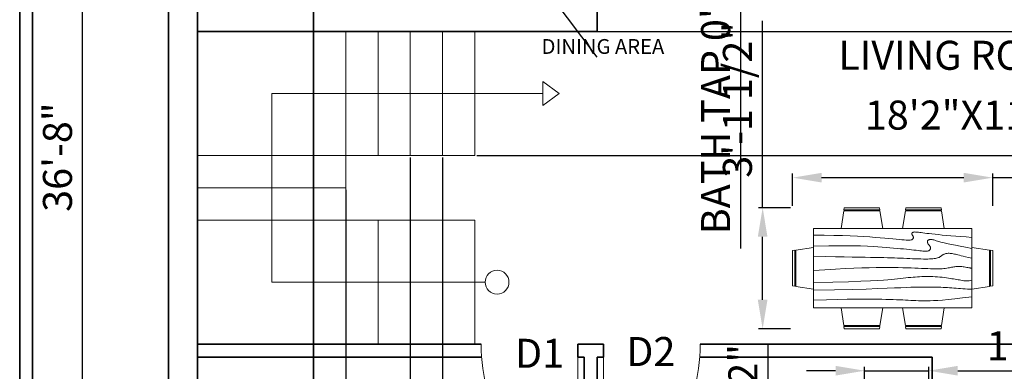
# Model space of a CAD drawing. Units: inches. Extents: x 2436 to 3928, y 1526 to 2149.
# Tile 2 of 6: x 2436 to 2742, y 1731 to 1840. Entities that reach past the tile are written whole.
import ezdxf

# ---------------------------------------------------------------- set-up
doc = ezdxf.new("R2010")
doc.units = ezdxf.units.IN
for name, color, linetype, lineweight in [('A-ANNO-SYMB', 7, 'Continuous', 13), ('A-AREA-IDEN', 152, 'Continuous', 18), ('A-DOOR', 4, 'Continuous', 18), ('A-DOOR-TEXT', 30, 'Continuous', 18), ('A-FLOR-STRS', 7, 'Continuous', 18), ('A-FURN', 8, 'Continuous', 18), ('A-WALL', 7, 'Continuous', 35), ('G-ANNO-TTLB', 7, 'Continuous', 35), ('S-ANNO-DIMS', 2, 'Continuous', 18)]:
    doc.layers.add(name, color=color, linetype=linetype, lineweight=lineweight)
doc.styles.get("Standard").update_dxf_attribs({"font": 'arial.ttf'})
doc.dimstyles.new('ISO-25', dxfattribs={"dimtxt": 9, "dimasz": 9, "dimexe": 1.25, "dimexo": 0.625, "dimgap": 2, "dimtad": 1, "dimdec": 1, "dimlunit": 4, "dimtxsty": 'Standard', "dimcen": 2.5, "dimadec": 0, "dimazin": 0, "dimtfac": 1, "dimtdec": 1, "dimtmove": 0, "dimatfit": 3, "dimfxl": 1, "dimarcsym": 0})

# ---------------------------------------------------------------- blocks, each defined once
blk = doc.blocks.new('Dining Set - 36 x 72 in.')
for p, q in [((-22, 27.5), (-22.1562, 26.50042)), ((-22, 27.5), (-6, 27.5)), ((-5.8437, 26.49966), (-6, 27.5)), ((6, 27.5), (5.8438, 26.50042)), ((6, 27.5), (22, 27.5)), ((22.1563, 26.49966), (22, 27.5)), ((-22.2343, 26.00059), (-23.4847, 17.99762)), ((-22.2304, 26), (-5.7608, 26)), ((-5.8416, 26.5), (-22.1534, 26.5)), ((-4.5152, 17.99762), (-5.7655, 25.99926)), ((5.7657, 26.00059), (4.5153, 17.99762)), ((5.7696, 26), (22.2392, 26)), ((22.1584, 26.5), (5.8466, 26.5)), ((23.4848, 17.99762), (22.2345, 25.99926)), ((36, 18), (-36, 18)), ((-36, 18), (-36, -18)), ((36, -18), (36, 18)), ((-44.0006, 8.23428), (-35.9976, 9.48474)), ((44.0006, 8.23428), (35.9976, 9.48474)), ((-45.5, 8), (-44.5004, 8.15617)), ((-45.5, 8), (-45.5, -8)), ((-44.5, -8.15843), (-44.5, 8.15338)), ((-44, 8.23041), (-44, -8.23915)), ((44, 8.23041), (44, -8.23915)), ((44.5, -8.15843), (44.5, 8.15338)), ((45.5, 8), (44.5005, 8.15617)), ((45.5, 8), (45.5, -8)), ((-44.4997, -8.15631), (-45.5, -8)), ((-35.9976, -9.48476), (-43.9993, -8.2345)), ((35.9976, -9.48476), (43.9993, -8.2345)), ((44.4997, -8.15631), (45.5, -8)), ((-36, -18), (36, -18)), ((-22.2343, -26.0006), (-23.4847, -17.99762)), ((-4.5152, -17.99762), (-5.7655, -25.99928)), ((5.7657, -26.0006), (4.5153, -17.99762)), ((23.4848, -17.99762), (22.2345, -25.99928)), ((-22.2304, -26), (-5.7608, -26)), ((-22, -27.5), (-22.1562, -26.50044)), ((-5.8416, -26.5), (-22.1534, -26.5)), ((-5.8437, -26.49967), (-6, -27.5)), ((5.7696, -26), (22.2392, -26)), ((6, -27.5), (5.8438, -26.50044)), ((22.1584, -26.5), (5.8466, -26.5)), ((22.1563, -26.49967), (22, -27.5)), ((-22, -27.5), (-6, -27.5)), ((6, -27.5), (22, -27.5))]:
    blk.add_line(p, q)
for points in [[(-36, 15), (-31.1772, 14.97754), (-26.8079, 14.91406), (-22.8538, 14.81543), (-19.276, 14.6875), (-16.0362, 14.53613), (-13.0957, 14.36718), (-10.4159, 14.18652), (-7.9583, 14), (-5.6904, 13.81315), (-3.6035, 13.63021), (-1.6954, 13.45508), (0.0365, 13.29166), (1.5945, 13.14388), (2.9811, 13.01562), (4.1988, 12.9108), (5.25, 12.83333), (6.1393, 12.78613), (6.8802, 12.76823), (7.4883, 12.77767), (7.9792, 12.8125), (8.3685, 12.87077), (8.6719, 12.95052), (8.9049, 13.0498), (9.0833, 13.16666), (9.2205, 13.29899), (9.3216, 13.44401), (9.3895, 13.59879), (9.4271, 13.76041), (9.4373, 13.92594), (9.4232, 14.09245), (9.3875, 14.257), (9.3333, 14.41666), (9.2638, 14.56917), (9.1836, 14.71484), (9.0975, 14.85465), (9.0104, 14.98958), (8.9272, 15.1206), (8.8529, 15.2487), (8.7922, 15.37483), (8.75, 15.5), (8.7305, 15.62467), (8.7344, 15.74739), (8.7617, 15.86621), (8.8125, 15.97916), (8.8867, 16.08431), (8.9844, 16.17968), (9.1055, 16.26334), (9.25, 16.33333), (9.4189, 16.38802), (9.6172, 16.42708), (9.8506, 16.45052), (10.125, 16.45833), (10.4463, 16.45052), (10.8203, 16.42708), (11.2529, 16.38802), (11.75, 16.33333), (12.3184, 16.26318), (12.9694, 16.17838), (13.7151, 16.07991), (14.5677, 15.96875), (15.5395, 15.84586), (16.6426, 15.71224), (17.8893, 15.56884), (19.2917, 15.41666), (20.859, 15.25667), (22.5879, 15.08984), (24.4721, 14.91715), (26.5052, 14.73958), (28.6809, 14.5581), (30.9929, 14.3737), (33.4347, 14.18733), (36, 14)], [(-36, 10), (-28.9766, 10.14274), (-23.1725, 10.20442), (-18.4241, 10.19775), (-14.5677, 10.13541), (-11.4399, 10.03011), (-8.877, 9.89453), (-6.7154, 9.74137), (-4.7917, 9.58333), (-2.9698, 9.43082), (-1.2246, 9.28515), (0.4415, 9.14534), (2.026, 9.01041), (3.5266, 8.87939), (4.9408, 8.7513), (6.266, 8.62516), (7.5, 8.5), (8.6411, 8.37549), (9.6914, 8.2539), (10.6538, 8.13818), (11.5312, 8.03125), (12.3267, 7.93603), (13.043, 7.85547), (13.6831, 7.79248), (14.25, 7.75), (14.7471, 7.7303), (15.1797, 7.73307), (15.5537, 7.75732), (15.875, 7.80208), (16.1494, 7.86637), (16.3828, 7.94922), (16.5811, 8.04964), (16.75, 8.16666), (16.8944, 8.29915), (17.0143, 8.44531), (17.1089, 8.60319), (17.1771, 8.77083), (17.218, 8.94629), (17.2305, 9.1276), (17.2137, 9.31282), (17.1667, 9.5), (17.0895, 9.6875), (16.987, 9.875), (16.8649, 10.0625), (16.7292, 10.25), (16.5856, 10.4375), (16.4401, 10.625), (16.2985, 10.8125), (16.1667, 11), (16.05, 11.18733), (15.9518, 11.3737), (15.8752, 11.5581), (15.8229, 11.73958), (15.798, 11.91715), (15.8034, 12.08984), (15.842, 12.25667), (15.9167, 12.41666), (16.0295, 12.56836), (16.1784, 12.70833), (16.3605, 12.83268), (16.5729, 12.9375), (16.8127, 13.01888), (17.0768, 13.07291), (17.3625, 13.0957), (17.6667, 13.08333), (17.9894, 13.03312), (18.3418, 12.94726), (18.7382, 12.82918), (19.1927, 12.68229), (19.7195, 12.51001), (20.3327, 12.31575), (21.0465, 12.10294), (21.875, 11.875), (22.8357, 11.63354), (23.959, 11.37304), (25.2786, 11.08618), (26.8282, 10.76562), (28.6414, 10.40405), (30.752, 9.99414), (33.1936, 9.52856), (36, 9)], [(-36, 5.5), (-30.7157, 5.3348), (-26.069, 5.20963), (-21.9946, 5.11767), (-18.4271, 5.05208), (-15.3009, 5.00602), (-12.5508, 4.97265), (-10.1112, 4.94515), (-7.9167, 4.91666), (-5.909, 4.88167), (-4.0586, 4.83984), (-2.3429, 4.79215), (-0.7396, 4.73958), (0.7739, 4.6831), (2.22, 4.6237), (3.6213, 4.56233), (5, 4.5), (6.373, 4.43782), (7.7344, 4.3776), (9.0723, 4.32129), (10.375, 4.27083), (11.6309, 4.22819), (12.8281, 4.19531), (13.9551, 4.17415), (15, 4.16666), (15.954, 4.17448), (16.819, 4.19791), (17.6001, 4.23698), (18.3021, 4.29166), (18.9299, 4.36198), (19.4883, 4.44791), (19.9823, 4.54948), (20.4167, 4.66666), (20.7969, 4.79899), (21.1302, 4.94401), (21.4245, 5.09879), (21.6875, 5.26041), (21.9271, 5.42594), (22.1511, 5.59245), (22.3672, 5.757), (22.5834, 5.91666), (22.8065, 6.06868), (23.0404, 6.21093), (23.2879, 6.34147), (23.5521, 6.45833), (23.8358, 6.55957), (24.142, 6.64323), (24.4735, 6.70735), (24.8334, 6.75), (25.2235, 6.76969), (25.642, 6.76692), (26.0858, 6.74267), (26.5521, 6.69791), (27.0379, 6.63362), (27.5404, 6.55078), (28.0565, 6.45036), (28.5834, 6.33333), (29.1242, 6.19987), (29.7071, 6.04687), (30.3661, 5.87044), (31.1354, 5.66666), (32.0493, 5.43164), (33.142, 5.16146), (34.4475, 4.85221), (36, 4.5)], [(-36, -1), (-30.7915, -0.6591), (-26.0195, -0.38216), (-21.6519, -0.16284), (-17.6563, 0.00521), (-14.0005, 0.12833), (-10.6523, 0.21289), (-7.5796, 0.26522), (-4.75, 0.29166), (-2.134, 0.29793), (0.2878, 0.28711), (2.5317, 0.26163), (4.6146, 0.22396), (6.5529, 0.17651), (8.3633, 0.12174), (10.0623, 0.06209), (11.6667, 0), (13.1899, -0.06201), (14.6341, -0.1211), (15.9982, -0.17432), (17.2813, -0.21875), (18.4823, -0.25147), (19.6003, -0.26953), (20.6343, -0.27002), (21.5834, -0.25), (22.4481, -0.20768), (23.2357, -0.14584), (23.9549, -0.06836), (24.6146, 0.02083), (25.2235, 0.11784), (25.7904, 0.21875), (26.3241, 0.31966), (26.8334, 0.41666), (27.3265, 0.50618), (27.8099, 0.58593), (28.2894, 0.65397), (28.7709, 0.70833), (29.2601, 0.74707), (29.763, 0.76823), (30.2855, 0.76985), (30.8334, 0.75), (31.4088, 0.70784), (31.9994, 0.64713), (32.589, 0.57275), (33.1615, 0.48958), (33.7008, 0.4025), (34.1908, 0.3164), (34.6153, 0.23616), (34.9584, 0.16666), (35.2099, 0.11165), (35.3848, 0.07031), (35.504, 0.04069), (35.5886, 0.02083), (35.6594, 0.00879), (35.7377, 0.0026), (35.8442, 0.00032), (36, 0)], [(-36, -6.5), (-27.1843, -6.31267), (-20.084, -6.1263), (-14.469, -5.9419), (-10.1094, -5.76042), (-6.7752, -5.58285), (-4.2363, -5.41016), (-2.2629, -5.24333), (-0.625, -5.08334), (0.8708, -4.93099), (2.2715, -4.78646), (3.5872, -4.64974), (4.8281, -4.52084), (6.0046, -4.39974), (7.127, -4.28646), (8.2053, -4.18099), (9.25, -4.08334), (10.2705, -3.99382), (11.2734, -3.91407), (12.2647, -3.84603), (13.25, -3.79167), (14.2354, -3.75293), (15.2266, -3.73177), (16.2295, -3.73015), (17.25, -3.75), (18.2912, -3.79248), (19.3451, -3.85547), (20.4009, -3.93604), (21.4479, -4.03125), (22.4754, -4.13819), (23.4727, -4.25391), (24.4289, -4.37549), (25.3334, -4.5), (26.1785, -4.62492), (26.9694, -4.74935), (27.7145, -4.87281), (28.4219, -4.99479), (29.1, -5.11483), (29.7572, -5.23242), (30.4016, -5.34709), (31.0417, -5.45834), (31.6837, -5.56437), (32.3262, -5.65821), (32.9658, -5.73153), (33.599, -5.77604), (34.2224, -5.78345), (34.8327, -5.74545), (35.4264, -5.65373), (36, -5.5)], [(-36, -10), (-26.4022, -9.81299), (-18.4675, -9.62891), (-11.9839, -9.45069), (-6.7396, -9.28125), (-2.5226, -9.12354), (0.8789, -8.98047), (3.6769, -8.85498), (6.0833, -8.75), (8.2767, -8.66765), (10.3021, -8.60677), (12.1712, -8.56543), (13.8958, -8.54167), (15.4876, -8.53353), (16.9583, -8.53907), (18.3197, -8.55632), (19.5834, -8.58334), (20.7616, -8.61841), (21.8685, -8.66081), (22.9188, -8.71004), (23.9271, -8.76563), (24.9081, -8.82707), (25.8763, -8.89388), (26.8465, -8.96558), (27.8334, -9.04167), (28.8474, -9.12118), (29.8828, -9.20117), (30.93, -9.27824), (31.9792, -9.34896), (33.0205, -9.40991), (34.0443, -9.45768), (35.0407, -9.48885), (36, -9.5)], [(-36, -14.5), (-30.0881, -14.33513), (-25.0332, -14.21224), (-20.7312, -14.12647), (-17.0781, -14.07292), (-13.97, -14.04671), (-11.3027, -14.04297), (-8.9724, -14.05681), (-6.875, -14.08334), (-4.9224, -14.11833), (-3.0905, -14.16016), (-1.3709, -14.20785), (0.2448, -14.26042), (1.7647, -14.3169), (3.1973, -14.3763), (4.5507, -14.43767), (5.8333, -14.5), (7.0554, -14.5621), (8.235, -14.62175), (9.3922, -14.67652), (10.5469, -14.72396), (11.7192, -14.76164), (12.929, -14.78711), (14.1965, -14.79794), (15.5417, -14.79167), (16.9933, -14.76424), (18.6152, -14.70508), (20.4804, -14.60197), (22.6615, -14.44271), (25.2312, -14.21509), (28.2624, -13.9069), (31.8277, -13.50594), (36, -13)]]:
    blk.add_lwpolyline(points)
blk = doc.blocks.new('DOOR-SINGLE-30-PLAN')
blk.add_line((0, 0), (0, 48))
blk.add_arc((-23.4, 0), 53.4, 0, 64.0108)
blk = doc.blocks.new('*D42')
at = {"layer": 'Defpoints', "color": 0, "transparency": 16777216}
for p in [(2658.27, 1927.9), (2658.27, 1917.9), (2659.77, 1917.9)]:
    blk.add_point(p, dxfattribs=at)
at = {"layer": 'S-ANNO-DIMS', "color": 0, "lineweight": -2, "transparency": 16777216}
for p, q in [((2659.77, 1936.9), (2659.77, 1945.9)), ((2658.9, 1927.9), (2661.02, 1927.9)), ((2659.77, 1927.9), (2659.77, 1917.9)), ((2658.9, 1917.9), (2661.02, 1917.9)), ((2659.77, 1908.9), (2659.77, 1769.48))]:
    blk.add_line(p, q, dxfattribs=at)
at = {"layer": 'S-ANNO-DIMS', "color": 0, "transparency": 16777216}
for points in [[(2658.27, 1936.9), (2661.27, 1936.9), (2659.77, 1927.9)], [(2658.27, 1908.9), (2661.27, 1908.9), (2659.77, 1917.9)]]:
    blk.add_solid(points, dxfattribs=at)
at = {"layer": 'S-ANNO-DIMS', "color": 0, "transparency": 16777216, "insert": (2653.18, 1834.69), "char_height": 9, "attachment_point": 5, "rotation": 90}
blk.add_mtext('BATH TAP 0\'-10" TYP.', dxfattribs=at)
blk = doc.blocks.new('*D48')
at = {"layer": 'Defpoints', "color": 0, "transparency": 16777216}
for p in [(2738.03, 1791.43), (2675.93, 1782.12), (2738.03, 1782.12)]:
    blk.add_point(p, dxfattribs=at)
at = {"layer": 'S-ANNO-DIMS', "color": 0, "lineweight": -2, "transparency": 16777216}
for p, q in [((2675.93, 1782.74), (2675.93, 1792.68)), ((2684.93, 1791.43), (2729.03, 1791.43)), ((2738.03, 1782.74), (2738.03, 1792.68)), ((2738.03, 1791.43), (2849.95, 1791.43))]:
    blk.add_line(p, q, dxfattribs=at)
at = {"layer": 'S-ANNO-DIMS', "color": 0, "transparency": 16777216}
for points in [[(2684.93, 1792.93), (2684.93, 1789.93), (2675.93, 1791.43)], [(2729.03, 1792.93), (2729.03, 1789.93), (2738.03, 1791.43)]]:
    blk.add_solid(points, dxfattribs=at)
at = {"layer": 'S-ANNO-DIMS', "color": 0, "transparency": 16777216, "insert": (2798.49, 1798.08), "char_height": 9, "attachment_point": 5}
blk.add_mtext('DINING SET 5\'-2"', dxfattribs=at)
blk = doc.blocks.new('*D49')
at = {"layer": 'Defpoints', "color": 0, "transparency": 16777216}
for p in [(2666.62, 1782.12), (2675.93, 1782.12), (2675.93, 1744.58)]:
    blk.add_point(p, dxfattribs=at)
at = {"layer": 'S-ANNO-DIMS', "color": 0, "lineweight": -2, "transparency": 16777216}
for p, q in [((2666.62, 1782.12), (2666.62, 1840.01)), ((2675.31, 1782.12), (2665.37, 1782.12)), ((2666.62, 1753.58), (2666.62, 1773.12)), ((2675.31, 1744.58), (2665.37, 1744.58))]:
    blk.add_line(p, q, dxfattribs=at)
at = {"layer": 'S-ANNO-DIMS', "color": 0, "transparency": 16777216}
for points in [[(2665.12, 1773.12), (2668.12, 1773.12), (2666.62, 1782.12)], [(2665.12, 1753.58), (2668.12, 1753.58), (2666.62, 1744.58)]]:
    blk.add_solid(points, dxfattribs=at)
at = {"layer": 'S-ANNO-DIMS', "color": 0, "transparency": 16777216, "insert": (2659.96, 1815.56), "char_height": 9, "attachment_point": 5, "rotation": 90}
blk.add_mtext('3\'-1 1/2"', dxfattribs=at)
blk = doc.blocks.new('*D51')
at = {"layer": 'Defpoints', "color": 0, "transparency": 16777216}
for p in [(2664.4, 1675.79), (2668.31, 1675.79), (2664.4, 1653.19)]:
    blk.add_point(p, dxfattribs=at)
at = {"layer": 'S-ANNO-DIMS', "color": 0, "lineweight": -2, "transparency": 16777216}
for p, q in [((2668.31, 1675.79), (2668.31, 1739.83)), ((2665.03, 1675.79), (2669.56, 1675.79)), ((2668.31, 1662.19), (2668.31, 1666.79)), ((2665.03, 1653.19), (2669.56, 1653.19))]:
    blk.add_line(p, q, dxfattribs=at)
at = {"layer": 'S-ANNO-DIMS', "color": 0, "transparency": 16777216}
for points in [[(2666.81, 1666.79), (2669.81, 1666.79), (2668.31, 1675.79)], [(2666.81, 1662.19), (2669.81, 1662.19), (2668.31, 1653.19)]]:
    blk.add_solid(points, dxfattribs=at)
at = {"layer": 'S-ANNO-DIMS', "color": 0, "transparency": 16777216, "insert": (2661.66, 1712.31), "char_height": 9, "attachment_point": 5, "rotation": 90}
blk.add_mtext('1\'-10 1/2"', dxfattribs=at)
blk = doc.blocks.new('*D55')
at = {"layer": 'Defpoints', "color": 0, "transparency": 16777216}
for p in [(2718.2, 1731.57), (2698.27, 1727.86), (2718.2, 1727.86)]:
    blk.add_point(p, dxfattribs=at)
at = {"layer": 'S-ANNO-DIMS', "color": 0, "lineweight": -2, "transparency": 16777216}
for p, q in [((2689.27, 1731.57), (2680.27, 1731.57)), ((2698.27, 1728.48), (2698.27, 1732.82)), ((2698.27, 1731.57), (2718.2, 1731.57)), ((2718.2, 1728.48), (2718.2, 1732.82)), ((2727.2, 1731.57), (2763.27, 1731.57))]:
    blk.add_line(p, q, dxfattribs=at)
at = {"layer": 'S-ANNO-DIMS', "color": 0, "transparency": 16777216}
for points in [[(2689.27, 1733.07), (2689.27, 1730.07), (2698.27, 1731.57)], [(2727.2, 1733.07), (2727.2, 1730.07), (2718.2, 1731.57)]]:
    blk.add_solid(points, dxfattribs=at)
at = {"layer": 'S-ANNO-DIMS', "color": 0, "transparency": 16777216, "insert": (2749.73, 1738.16), "char_height": 9, "attachment_point": 5}
blk.add_mtext('1\'-8"', dxfattribs=at)
blk = doc.blocks.new('*D57')
at = {"layer": 'Defpoints', "color": 0, "transparency": 16777216}
for p in [(2455.49, 2017.79), (2482.24, 2017.79), (2482.24, 1577.79)]:
    blk.add_point(p, dxfattribs=at)
at = {"layer": 'S-ANNO-DIMS', "color": 0, "lineweight": -2, "transparency": 16777216}
for p, q in [((2481.61, 2017.79), (2454.24, 2017.79)), ((2455.49, 1586.79), (2455.49, 2008.79)), ((2481.61, 1577.79), (2454.24, 1577.79))]:
    blk.add_line(p, q, dxfattribs=at)
at = {"layer": 'S-ANNO-DIMS', "color": 0, "transparency": 16777216}
for points in [[(2453.99, 2008.79), (2456.99, 2008.79), (2455.49, 2017.79)], [(2453.99, 1586.79), (2456.99, 1586.79), (2455.49, 1577.79)]]:
    blk.add_solid(points, dxfattribs=at)
at = {"layer": 'S-ANNO-DIMS', "color": 0, "transparency": 16777216, "insert": (2448.89, 1797.79), "char_height": 9, "attachment_point": 5, "rotation": 90}
blk.add_mtext('36\'-8"', dxfattribs=at)
blk = doc.blocks.new('*D58')
at = {"layer": 'Defpoints', "color": 0, "transparency": 16777216}
for p in [(2491.24, 2008.79), (2527.24, 2008.79), (2527.24, 1551.04)]:
    blk.add_point(p, dxfattribs=at)
at = {"layer": 'S-ANNO-DIMS', "color": 0, "lineweight": -2, "transparency": 16777216}
for p, q in [((2491.24, 2008.16), (2491.24, 1549.79)), ((2527.24, 2008.16), (2527.24, 1549.79)), ((2500.24, 1551.04), (2518.24, 1551.04))]:
    blk.add_line(p, q, dxfattribs=at)
at = {"layer": 'S-ANNO-DIMS', "color": 0, "transparency": 16777216}
for points in [[(2500.24, 1552.54), (2500.24, 1549.54), (2491.24, 1551.04)], [(2518.24, 1552.54), (2518.24, 1549.54), (2527.24, 1551.04)]]:
    blk.add_solid(points, dxfattribs=at)
at = {"layer": 'S-ANNO-DIMS', "color": 0, "transparency": 16777216, "insert": (2509.24, 1557.64), "char_height": 9, "attachment_point": 5}
blk.add_mtext('3\'-0"', dxfattribs=at)
blk = doc.blocks.new('*D64')
at = {"layer": 'Defpoints', "color": 0, "transparency": 16777216}
for p in [(2527.24, 2114.67), (2491.24, 1603.79), (2527.24, 1603.79)]:
    blk.add_point(p, dxfattribs=at)
at = {"layer": 'S-ANNO-DIMS', "color": 0, "lineweight": -2, "transparency": 16777216}
for p, q in [((2491.24, 1604.41), (2491.24, 2115.92)), ((2527.24, 1604.41), (2527.24, 2115.92)), ((2500.24, 2114.67), (2518.24, 2114.67))]:
    blk.add_line(p, q, dxfattribs=at)
at = {"layer": 'S-ANNO-DIMS', "color": 0, "transparency": 16777216}
for points in [[(2500.24, 2116.17), (2500.24, 2113.17), (2491.24, 2114.67)], [(2518.24, 2116.17), (2518.24, 2113.17), (2527.24, 2114.67)]]:
    blk.add_solid(points, dxfattribs=at)
at = {"layer": 'S-ANNO-DIMS', "color": 0, "transparency": 16777216, "insert": (2509.24, 2121.27), "char_height": 9, "attachment_point": 5}
blk.add_mtext('3\'-0"', dxfattribs=at)
blk = doc.blocks.new('*D71')
at = {"layer": 'Defpoints', "color": 0, "transparency": 16777216}
for p in [(2577.24, 1836.79), (2868.99, 1836.79), (2577.24, 1798.29)]:
    blk.add_point(p, dxfattribs=at)
at = {"layer": 'S-ANNO-DIMS', "color": 0, "lineweight": -2, "transparency": 16777216}
for p, q in [((2868.99, 1836.79), (2868.99, 1894.68)), ((2577.86, 1836.79), (2870.24, 1836.79)), ((2868.99, 1807.29), (2868.99, 1827.79)), ((2577.86, 1798.29), (2870.24, 1798.29))]:
    blk.add_line(p, q, dxfattribs=at)
at = {"layer": 'S-ANNO-DIMS', "color": 0, "transparency": 16777216}
for points in [[(2867.49, 1827.79), (2870.49, 1827.79), (2868.99, 1836.79)], [(2867.49, 1807.29), (2870.49, 1807.29), (2868.99, 1798.29)]]:
    blk.add_solid(points, dxfattribs=at)
at = {"layer": 'S-ANNO-DIMS', "color": 0, "transparency": 16777216, "insert": (2862.33, 1870.23), "char_height": 9, "attachment_point": 5, "rotation": 90}
blk.add_mtext('3\'-2 1/2"', dxfattribs=at)
blk = doc.blocks.new('*D72')
at = {"layer": 'Defpoints', "color": 0, "transparency": 16777216}
for p in [(2491.24, 1798.29), (2537.24, 1788.29), (2537.24, 1551.04)]:
    blk.add_point(p, dxfattribs=at)
at = {"layer": 'S-ANNO-DIMS', "color": 0, "lineweight": -2, "transparency": 16777216}
for p, q in [((2491.24, 1797.66), (2491.24, 1549.79)), ((2537.24, 1787.66), (2537.24, 1549.79)), ((2500.24, 1551.04), (2528.24, 1551.04))]:
    blk.add_line(p, q, dxfattribs=at)
at = {"layer": 'S-ANNO-DIMS', "color": 0, "transparency": 16777216}
for points in [[(2500.24, 1552.54), (2500.24, 1549.54), (2491.24, 1551.04)], [(2528.24, 1552.54), (2528.24, 1549.54), (2537.24, 1551.04)]]:
    blk.add_solid(points, dxfattribs=at)
at = {"layer": 'S-ANNO-DIMS', "color": 0, "transparency": 16777216, "insert": (2514.24, 1557.64), "char_height": 9, "attachment_point": 5}
blk.add_mtext('3\'-10"', dxfattribs=at)
blk = doc.blocks.new('*D73')
at = {"layer": 'Defpoints', "color": 0, "transparency": 16777216}
for p in [(2557.24, 1798.29), (2567.24, 1798.29), (2567.24, 1551.04)]:
    blk.add_point(p, dxfattribs=at)
at = {"layer": 'S-ANNO-DIMS', "color": 0, "lineweight": -2, "transparency": 16777216}
for p, q in [((2557.24, 1797.66), (2557.24, 1549.79)), ((2567.24, 1797.66), (2567.24, 1549.79)), ((2548.24, 1551.04), (2539.24, 1551.04)), ((2557.24, 1551.04), (2567.24, 1551.04)), ((2576.24, 1551.04), (2620.16, 1551.04))]:
    blk.add_line(p, q, dxfattribs=at)
at = {"layer": 'S-ANNO-DIMS', "color": 0, "transparency": 16777216}
for points in [[(2548.24, 1552.54), (2548.24, 1549.54), (2557.24, 1551.04)], [(2576.24, 1552.54), (2576.24, 1549.54), (2567.24, 1551.04)]]:
    blk.add_solid(points, dxfattribs=at)
at = {"layer": 'S-ANNO-DIMS', "color": 0, "transparency": 16777216, "insert": (2602.7, 1557.63), "char_height": 9, "attachment_point": 5}
blk.add_mtext('0\'-10"', dxfattribs=at)
blk = doc.blocks.new('*D83')
at = {"layer": 'Defpoints', "color": 0, "transparency": 16777216}
for p in [(2585.24, 1868.79), (2615.24, 1828.79)]:
    blk.add_point(p, dxfattribs=at)
at = {"layer": 'S-ANNO-DIMS', "color": 0, "lineweight": -2, "transparency": 16777216}
for p, q in [((2552.51, 1912.42), (2579.84, 1875.99)), ((2615.24, 1828.79), (2585.24, 1868.79))]:
    blk.add_line(p, q, dxfattribs=at)
at = {"layer": 'S-ANNO-DIMS', "color": 0, "transparency": 16777216}
blk.add_solid([(2581.04, 1876.89), (2578.64, 1875.09), (2585.24, 1868.79)], dxfattribs=at)
at = {"layer": 'S-ANNO-DIMS', "color": 0, "transparency": 16777216, "insert": (2568.69, 1901.72), "char_height": 9, "attachment_point": 5, "rotation": 306.8705}
blk.add_mtext('R4\'-2"', dxfattribs=at)

msp = doc.modelspace()

# ---------------------------------------------------------------- linework, layer by layer
at = {"layer": 'A-ANNO-SYMB'}
for p, q in [((2598.42, 1817.54), (2598.42, 1821.24)), ((2598.42, 1821.24), (2603.42, 1817.54)), ((2514.24, 1759.02), (2514.24, 1817.54)), ((2514.24, 1817.54), (2598.42, 1817.54)), ((2598.42, 1817.54), (2598.42, 1813.84)), ((2598.42, 1813.84), (2603.42, 1817.54)), ((2580.47, 1759.02), (2514.24, 1759.02))]:
    msp.add_line(p, q, dxfattribs=at)
msp.add_circle((2584.17, 1759.02), 3.7, dxfattribs=at)
at = {"layer": 'A-FLOR-STRS'}
for p, q in [((2537.24, 1739.79), (2537.24, 1836.79)), ((2547.24, 1798.29), (2547.24, 1836.79)), ((2557.24, 1798.29), (2557.24, 1836.79)), ((2567.24, 1798.29), (2567.24, 1836.79)), ((2577.24, 1798.29), (2577.24, 1836.79)), ((2491.24, 1798.29), (2577.24, 1798.29)), ((2491.24, 1788.29), (2537.24, 1788.29)), ((2491.24, 1778.29), (2577.24, 1778.29)), ((2547.24, 1739.79), (2547.24, 1778.29)), ((2557.24, 1739.79), (2557.24, 1778.29)), ((2567.24, 1739.79), (2567.24, 1778.29)), ((2577.24, 1739.79), (2577.24, 1778.29))]:
    msp.add_line(p, q, dxfattribs=at)
at = {"layer": 'A-WALL'}
for p, q in [((2482.24, 1577.79), (2482.24, 2017.79)), ((2615.24, 1836.79), (2615.24, 1842.79)), ((2491.24, 1836.79), (2615.24, 1836.79)), ((2491.24, 1739.79), (2491.24, 1836.79)), ((2491.24, 1739.79), (2579.24, 1739.79)), ((2609.24, 1735.79), (2609.24, 1739.79)), ((2609.24, 1739.79), (2617.24, 1739.79)), ((2609.24, 1735.79), (2609.24, 1739.79)), ((2615.24, 1739.79), (2617.24, 1739.79)), ((2617.24, 1735.79), (2617.24, 1739.79)), ((2647.24, 1739.79), (2783.24, 1739.79)), ((2491.24, 1735.79), (2579.39, 1735.79)), ((2491.24, 1615.79), (2491.24, 1735.79)), ((2609.24, 1735.79), (2611.24, 1735.79)), ((2611.24, 1615.79), (2611.24, 1735.79)), ((2615.24, 1651.79), (2615.24, 1735.79)), ((2615.24, 1735.79), (2617.24, 1735.79)), ((2647.09, 1735.79), (2719.24, 1735.79)), ((2719.24, 1651.79), (2719.24, 1735.79))]:
    msp.add_line(p, q, dxfattribs=at)
at = {"layer": 'G-ANNO-TTLB'}
for points in [[(2436, 2138.4), (3927.51, 2138.4), (3927.51, 1525.6), (2436, 1525.6)], [(2440, 2134.4), (3923.51, 2134.4), (3923.51, 1529.6), (2440, 1529.6)]]:
    msp.add_lwpolyline(points, close=True, dxfattribs=at)

# ---------------------------------------------------------------- block references
at = {"layer": 'A-DOOR', "rotation": 180}
msp.add_blockref('DOOR-SINGLE-30-PLAN', (2609.24, 1739.79), dxfattribs=at)
at = {"layer": 'A-DOOR', "extrusion": (0, 0, -1), "zscale": -1, "rotation": 180}
msp.add_blockref('DOOR-SINGLE-30-PLAN', (-2617.24, 1739.79), dxfattribs=at)
at = {"layer": 'A-FURN', "xscale": 0.6824034264036987, "yscale": 0.6824034264036987, "zscale": 0.6824034264036987}
msp.add_blockref('Dining Set - 36 x 72 in.', (2706.98, 1763.35), dxfattribs=at)

# ---------------------------------------------------------------- texts
at = {"layer": 'A-AREA-IDEN'}
for s, height, p in [('DINING AREA', 4.5967, (2598, 1829.8)), ('LIVING ROOM', 9, (2690.1, 1824.87)), ('   18\'2"X11\'8"', 9, (2690.1, 1806.33))]:
    msp.add_text(s, height=height, dxfattribs=at).set_placement(p)
at = {"layer": 'A-DOOR-TEXT'}
for s, p in [('D2', (2624.27, 1733.02)), ('D1', (2589.74, 1732.47))]:
    msp.add_text(s, height=9, dxfattribs=at).set_placement(p)

# ---------------------------------------------------------------- dimensions: what is measured, and where the dimension line sits
at = {"layer": 'S-ANNO-DIMS'}
for base, p1, p2, picture, middle in [((2527.24, 2114.67), (2491.24, 1603.79), (2527.24, 1603.79), '*D64', (2509.24, 2121.27)), ((2527.24, 1551.04), (2491.24, 2008.79), (2527.24, 2008.79), '*D58', (2509.24, 1557.64)), ((2537.24, 1551.04), (2491.24, 1798.29), (2537.24, 1788.29), '*D72', (2514.24, 1557.64)), ((2567.24, 1551.04), (2557.24, 1798.29), (2567.24, 1798.29), '*D73', (2602.7, 1557.63)), ((2718.2, 1731.57), (2698.27, 1727.86), (2718.2, 1727.86), '*D55', (2749.73, 1738.16))]:
    dim = msp.add_linear_dim(base=base, p1=p1, p2=p2, dimstyle='ISO-25', override={"dimdec": 1, "dimlfac": 1, "dimrnd": 0, "dimzin": 1, "dimdsep": 46, "dimlunit": 4, "dimfrac": 2}, dxfattribs=at)
    dim.commit()
    dim.dimension.update_dxf_attribs({"geometry": picture, "text_midpoint": middle})
for base, p1, p2, picture, middle in [((2455.49, 2017.79), (2482.24, 1577.79), (2482.24, 2017.79), '*D57', (2448.89, 1797.79)), ((2868.99, 1836.79), (2577.24, 1798.29), (2577.24, 1836.79), '*D71', (2862.33, 1870.23)), ((2666.62, 1782.12), (2675.93, 1744.58), (2675.93, 1782.12), '*D49', (2659.96, 1815.56)), ((2668.31, 1675.79), (2664.4, 1653.19), (2664.4, 1675.79), '*D51', (2661.66, 1712.31))]:
    dim = msp.add_linear_dim(base=base, p1=p1, p2=p2, angle=90, dimstyle='ISO-25', override={"dimdec": 1, "dimlfac": 1, "dimrnd": 0, "dimzin": 1, "dimdsep": 46, "dimlunit": 4, "dimfrac": 2}, dxfattribs=at)
    dim.commit()
    dim.dimension.update_dxf_attribs({"geometry": picture, "text_midpoint": middle})
dim = msp.add_linear_dim(base=(2659.77, 1917.9), p1=(2658.27, 1927.9), p2=(2658.27, 1917.9), angle=270, text='BATH TAP <> TYP.', dimstyle='ISO-25', override={"dimdec": 1, "dimlfac": 1, "dimrnd": 0, "dimzin": 1, "dimdsep": 46, "dimlunit": 4, "dimfrac": 2}, dxfattribs=at)
dim.commit()
dim.dimension.update_dxf_attribs({"geometry": '*D42', "text_midpoint": (2653.18, 1834.69)})
dim = msp.add_radius_dim(center=(2615.24, 1828.79), mpoint=(2585.24, 1868.79), dimstyle='ISO-25', override={"dimdec": 1, "dimlfac": 1, "dimrnd": 0, "dimzin": 1, "dimdsep": 46, "dimlunit": 4, "dimfrac": 2}, dxfattribs=at)
dim.commit()
dim.dimension.update_dxf_attribs({"geometry": '*D83', "text_midpoint": (2568.69, 1901.72)})
dim = msp.add_linear_dim(base=(2738.03, 1791.43), p1=(2675.93, 1782.12), p2=(2738.03, 1782.12), text='DINING SET <>', dimstyle='ISO-25', override={"dimdec": 1, "dimlfac": 1, "dimrnd": 0, "dimzin": 1, "dimdsep": 46, "dimlunit": 4, "dimfrac": 2}, dxfattribs=at)
dim.commit()
dim.dimension.update_dxf_attribs({"geometry": '*D48', "text_midpoint": (2798.49, 1798.08)})

doc.saveas('drawing.dxf')
